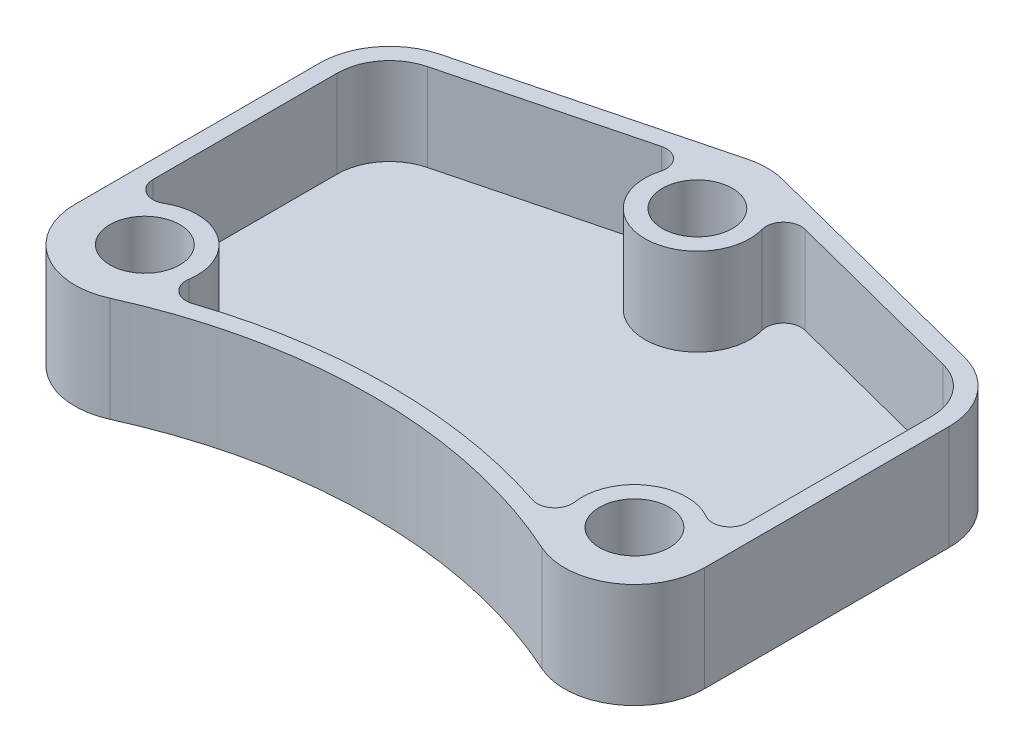
ISO-10303-21;
HEADER;
FILE_DESCRIPTION(('STEP AP214'),'2;1');
FILE_NAME('part.step','',(''),(''),'','','');
FILE_SCHEMA(('AUTOMOTIVE_DESIGN { 1 0 10303 214 1 1 1 1 }'));
ENDSEC;
DATA;
#1=APPLICATION_CONTEXT('core data for automotive mechanical design processes');
#2=APPLICATION_PROTOCOL_DEFINITION('international standard','automotive_design',2000,#1);
#3=PRODUCT_CONTEXT('',#1,'mechanical');
#4=PRODUCT('Part','Part','',(#3));
#5=PRODUCT_RELATED_PRODUCT_CATEGORY('part','',(#4));
#6=PRODUCT_DEFINITION_FORMATION('','',#4);
#7=PRODUCT_DEFINITION_CONTEXT('part definition',#1,'design');
#8=PRODUCT_DEFINITION('design','',#6,#7);
#9=PRODUCT_DEFINITION_SHAPE('','',#8);
#10=(LENGTH_UNIT() NAMED_UNIT(*) SI_UNIT(.MILLI.,.METRE.));
#11=(NAMED_UNIT(*) PLANE_ANGLE_UNIT() SI_UNIT($,.RADIAN.));
#12=(NAMED_UNIT(*) SI_UNIT($,.STERADIAN.) SOLID_ANGLE_UNIT());
#13=UNCERTAINTY_MEASURE_WITH_UNIT(LENGTH_MEASURE(1.E-05),#10,'distance_accuracy_value','');
#14=(GEOMETRIC_REPRESENTATION_CONTEXT(3) GLOBAL_UNCERTAINTY_ASSIGNED_CONTEXT((#13)) GLOBAL_UNIT_ASSIGNED_CONTEXT((#10,
#11,#12)) REPRESENTATION_CONTEXT('',''));
#15=CARTESIAN_POINT('',(0.,0.,0.));
#16=DIRECTION('',(0.,0.,1.));
#17=DIRECTION('',(1.,0.,0.));
#18=AXIS2_PLACEMENT_3D('',#15,#16,#17);
#19=CARTESIAN_POINT('',(-70.,30.,18.));
#20=DIRECTION('',(0.,1.,0.));
#21=DIRECTION('',(0.,0.,1.));
#22=AXIS2_PLACEMENT_3D('',#19,#20,#21);
#23=PLANE('',#22);
#24=CARTESIAN_POINT('',(70.,30.,88.));
#25=DIRECTION('',(0.,1.,0.));
#26=DIRECTION('',(0.,0.,1.));
#27=AXIS2_PLACEMENT_3D('',#24,#25,#26);
#28=CIRCLE('',#27,9.99999999999999);
#29=CARTESIAN_POINT('',(70.,30.,98.));
#30=VERTEX_POINT('',#29);
#31=EDGE_CURVE('E240',#30,#30,#28,.T.);
#32=ORIENTED_EDGE('',*,*,#31,.F.);
#33=EDGE_LOOP('',(#32));
#34=FACE_BOUND('',#33,.T.);
#35=CARTESIAN_POINT('',(0.,30.,0.));
#36=DIRECTION('',(0.,1.,0.));
#37=DIRECTION('',(0.,0.,1.));
#38=AXIS2_PLACEMENT_3D('',#35,#36,#37);
#39=CIRCLE('',#38,10.);
#40=CARTESIAN_POINT('',(0.,30.,10.));
#41=VERTEX_POINT('',#40);
#42=EDGE_CURVE('E163',#41,#41,#39,.T.);
#43=ORIENTED_EDGE('',*,*,#42,.F.);
#44=EDGE_LOOP('',(#43));
#45=FACE_BOUND('',#44,.T.);
#46=CARTESIAN_POINT('',(-70.,30.,18.));
#47=DIRECTION('',(0.,1.,0.));
#48=DIRECTION('',(0.,0.,1.));
#49=AXIS2_PLACEMENT_3D('',#46,#47,#48);
#50=CIRCLE('',#49,20.);
#51=CARTESIAN_POINT('',(-74.9808207962124,30.,-1.36985865193699));
#52=VERTEX_POINT('',#51);
#53=CARTESIAN_POINT('',(-90.,30.,18.));
#54=VERTEX_POINT('',#53);
#55=EDGE_CURVE('E179',#52,#54,#50,.T.);
#56=ORIENTED_EDGE('',*,*,#55,.T.);
#57=DIRECTION('',(0.,0.,1.));
#58=VECTOR('',#57,1.);
#59=CARTESIAN_POINT('',(-90.,30.,18.));
#60=LINE('',#59,#58);
#61=CARTESIAN_POINT('',(-90.,30.,88.));
#62=VERTEX_POINT('',#61);
#63=EDGE_CURVE('E109',#54,#62,#60,.T.);
#64=ORIENTED_EDGE('',*,*,#63,.T.);
#65=CARTESIAN_POINT('',(-70.,30.,88.));
#66=DIRECTION('',(0.,1.,0.));
#67=DIRECTION('',(0.,0.,1.));
#68=AXIS2_PLACEMENT_3D('',#65,#66,#67);
#69=CIRCLE('',#68,20.);
#70=CARTESIAN_POINT('',(-61.7647058823529,30.,106.225803982153));
#71=VERTEX_POINT('',#70);
#72=EDGE_CURVE('E203',#62,#71,#69,.T.);
#73=ORIENTED_EDGE('',*,*,#72,.T.);
#74=CARTESIAN_POINT('',(0.,30.,242.919333848297));
#75=DIRECTION('',(0.,-1.,0.));
#76=DIRECTION('',(0.,0.,-1.));
#77=AXIS2_PLACEMENT_3D('',#74,#75,#76);
#78=CIRCLE('',#77,150.);
#79=CARTESIAN_POINT('',(61.7647058823529,30.,106.225803982153));
#80=VERTEX_POINT('',#79);
#81=EDGE_CURVE('E219',#71,#80,#78,.T.);
#82=ORIENTED_EDGE('',*,*,#81,.T.);
#83=CARTESIAN_POINT('',(70.,30.,88.));
#84=DIRECTION('',(0.,1.,0.));
#85=DIRECTION('',(0.,0.,1.));
#86=AXIS2_PLACEMENT_3D('',#83,#84,#85);
#87=CIRCLE('',#86,20.);
#88=CARTESIAN_POINT('',(90.,30.,88.));
#89=VERTEX_POINT('',#88);
#90=EDGE_CURVE('E220',#80,#89,#87,.T.);
#91=ORIENTED_EDGE('',*,*,#90,.T.);
#92=DIRECTION('',(0.,0.,-1.));
#93=VECTOR('',#92,1.);
#94=CARTESIAN_POINT('',(90.,30.,18.));
#95=LINE('',#94,#93);
#96=CARTESIAN_POINT('',(90.,30.,18.));
#97=VERTEX_POINT('',#96);
#98=EDGE_CURVE('E218',#89,#97,#95,.T.);
#99=ORIENTED_EDGE('',*,*,#98,.T.);
#100=CARTESIAN_POINT('',(70.,30.,18.));
#101=DIRECTION('',(0.,1.,0.));
#102=DIRECTION('',(0.,0.,-1.));
#103=AXIS2_PLACEMENT_3D('',#100,#101,#102);
#104=CIRCLE('',#103,20.);
#105=CARTESIAN_POINT('',(74.9808207962124,30.,-1.36985865193699));
#106=VERTEX_POINT('',#105);
#107=EDGE_CURVE('E137',#97,#106,#104,.T.);
#108=ORIENTED_EDGE('',*,*,#107,.T.);
#109=DIRECTION('',(-0.96849293259685,0.,-0.249041039810618));
#110=VECTOR('',#109,1.);
#111=CARTESIAN_POINT('',(74.9808207962124,30.,-1.36985865193699));
#112=LINE('',#111,#110);
#113=CARTESIAN_POINT('',(4.98082079621237,30.,-19.369858651937));
#114=VERTEX_POINT('',#113);
#115=EDGE_CURVE('E135',#106,#114,#112,.T.);
#116=ORIENTED_EDGE('',*,*,#115,.T.);
#117=CARTESIAN_POINT('',(0.,30.,0.));
#118=DIRECTION('',(0.,1.,0.));
#119=DIRECTION('',(0.,0.,1.));
#120=AXIS2_PLACEMENT_3D('',#117,#118,#119);
#121=CIRCLE('',#120,20.);
#122=CARTESIAN_POINT('',(-4.98082079621237,30.,-19.369858651937));
#123=VERTEX_POINT('',#122);
#124=EDGE_CURVE('E138',#114,#123,#121,.T.);
#125=ORIENTED_EDGE('',*,*,#124,.T.);
#126=DIRECTION('',(-0.96849293259685,0.,0.249041039810618));
#127=VECTOR('',#126,1.);
#128=CARTESIAN_POINT('',(-74.9808207962124,30.,-1.36985865193699));
#129=LINE('',#128,#127);
#130=EDGE_CURVE('E64',#123,#52,#129,.T.);
#131=ORIENTED_EDGE('',*,*,#130,.T.);
#132=EDGE_LOOP('',(#56,#64,#73,#82,#91,#99,#108,#116,#125,#131));
#133=FACE_BOUND('',#132,.T.);
#134=CARTESIAN_POINT('',(-70.,30.,88.));
#135=DIRECTION('',(0.,1.,0.));
#136=DIRECTION('',(0.,0.,1.));
#137=AXIS2_PLACEMENT_3D('',#134,#135,#136);
#138=CIRCLE('',#137,9.99999999999999);
#139=CARTESIAN_POINT('',(-70.,30.,98.));
#140=VERTEX_POINT('',#139);
#141=EDGE_CURVE('E233',#140,#140,#138,.T.);
#142=ORIENTED_EDGE('',*,*,#141,.F.);
#143=EDGE_LOOP('',(#142));
#144=FACE_BOUND('',#143,.T.);
#145=CARTESIAN_POINT('',(19.2652000583974,30.,-5.37141198475075));
#146=DIRECTION('',(0.,1.,0.));
#147=DIRECTION('',(0.,0.,1.));
#148=AXIS2_PLACEMENT_3D('',#145,#146,#147);
#149=CIRCLE('',#148,5.);
#150=CARTESIAN_POINT('',(20.5104052574505,30.,-10.213876647735));
#151=VERTEX_POINT('',#150);
#152=CARTESIAN_POINT('',(14.4489000437981,30.,-4.02855898856307));
#153=VERTEX_POINT('',#152);
#154=EDGE_CURVE('E53',#151,#153,#149,.T.);
#155=ORIENTED_EDGE('',*,*,#154,.F.);
#156=DIRECTION('',(-0.96849293259685,0.,-0.249041039810618));
#157=VECTOR('',#156,1.);
#158=CARTESIAN_POINT('',(73.7356155971593,30.,3.47260601104726));
#159=LINE('',#158,#157);
#160=CARTESIAN_POINT('',(73.7356155971593,30.,3.47260601104726));
#161=VERTEX_POINT('',#160);
#162=EDGE_CURVE('E295',#161,#151,#159,.T.);
#163=ORIENTED_EDGE('',*,*,#162,.F.);
#164=CARTESIAN_POINT('',(70.,30.,18.));
#165=DIRECTION('',(0.,1.,0.));
#166=DIRECTION('',(0.,0.,1.));
#167=AXIS2_PLACEMENT_3D('',#164,#165,#166);
#168=CIRCLE('',#167,15.);
#169=CARTESIAN_POINT('',(85.,30.,18.));
#170=VERTEX_POINT('',#169);
#171=EDGE_CURVE('E297',#170,#161,#168,.T.);
#172=ORIENTED_EDGE('',*,*,#171,.F.);
#173=DIRECTION('',(0.,0.,-1.));
#174=VECTOR('',#173,1.);
#175=CARTESIAN_POINT('',(85.,30.,70.6794919243112));
#176=LINE('',#175,#174);
#177=CARTESIAN_POINT('',(85.,30.,70.6794919243112));
#178=VERTEX_POINT('',#177);
#179=EDGE_CURVE('E296',#178,#170,#176,.T.);
#180=ORIENTED_EDGE('',*,*,#179,.F.);
#181=CARTESIAN_POINT('',(80.,30.,70.6794919243112));
#182=DIRECTION('',(0.,1.,0.));
#183=DIRECTION('',(0.,0.,1.));
#184=AXIS2_PLACEMENT_3D('',#181,#182,#183);
#185=CIRCLE('',#184,5.00000000000001);
#186=CARTESIAN_POINT('',(77.5,30.,75.0096189432334));
#187=VERTEX_POINT('',#186);
#188=EDGE_CURVE('E305',#187,#178,#185,.T.);
#189=ORIENTED_EDGE('',*,*,#188,.F.);
#190=CARTESIAN_POINT('',(70.,30.,88.));
#191=DIRECTION('',(0.,-1.,0.));
#192=DIRECTION('',(0.,0.,1.));
#193=AXIS2_PLACEMENT_3D('',#190,#191,#192);
#194=CIRCLE('',#193,15.);
#195=CARTESIAN_POINT('',(55.1705641207694,30.,90.255622198815));
#196=VERTEX_POINT('',#195);
#197=EDGE_CURVE('E304',#196,#187,#194,.T.);
#198=ORIENTED_EDGE('',*,*,#197,.F.);
#199=CARTESIAN_POINT('',(50.2274188276925,30.,91.0074962650867));
#200=DIRECTION('',(0.,1.,0.));
#201=DIRECTION('',(0.,0.,1.));
#202=AXIS2_PLACEMENT_3D('',#199,#200,#201);
#203=CIRCLE('',#202,5.);
#204=CARTESIAN_POINT('',(48.6578119893271,30.,95.754741189562));
#205=VERTEX_POINT('',#204);
#206=EDGE_CURVE('E306',#205,#196,#203,.T.);
#207=ORIENTED_EDGE('',*,*,#206,.F.);
#208=CARTESIAN_POINT('',(0.,30.,242.919333848297));
#209=DIRECTION('',(0.,-1.,0.));
#210=DIRECTION('',(0.,0.,1.));
#211=AXIS2_PLACEMENT_3D('',#208,#209,#210);
#212=CIRCLE('',#211,155.);
#213=CARTESIAN_POINT('',(-48.657811989327,30.,95.754741189562));
#214=VERTEX_POINT('',#213);
#215=EDGE_CURVE('E313',#214,#205,#212,.T.);
#216=ORIENTED_EDGE('',*,*,#215,.F.);
#217=CARTESIAN_POINT('',(-50.2274188276925,30.,91.0074962650867));
#218=DIRECTION('',(0.,1.,0.));
#219=DIRECTION('',(0.,0.,1.));
#220=AXIS2_PLACEMENT_3D('',#217,#218,#219);
#221=CIRCLE('',#220,5.);
#222=CARTESIAN_POINT('',(-55.1705641207694,30.,90.255622198815));
#223=VERTEX_POINT('',#222);
#224=EDGE_CURVE('E314',#223,#214,#221,.T.);
#225=ORIENTED_EDGE('',*,*,#224,.F.);
#226=CARTESIAN_POINT('',(-70.,30.,88.));
#227=DIRECTION('',(0.,-1.,0.));
#228=DIRECTION('',(0.,0.,1.));
#229=AXIS2_PLACEMENT_3D('',#226,#227,#228);
#230=CIRCLE('',#229,15.);
#231=CARTESIAN_POINT('',(-77.5,30.,75.0096189432334));
#232=VERTEX_POINT('',#231);
#233=EDGE_CURVE('E320',#232,#223,#230,.T.);
#234=ORIENTED_EDGE('',*,*,#233,.F.);
#235=CARTESIAN_POINT('',(-80.,30.,70.6794919243112));
#236=DIRECTION('',(0.,1.,0.));
#237=DIRECTION('',(0.,0.,1.));
#238=AXIS2_PLACEMENT_3D('',#235,#236,#237);
#239=CIRCLE('',#238,5.);
#240=CARTESIAN_POINT('',(-85.,30.,70.6794919243112));
#241=VERTEX_POINT('',#240);
#242=EDGE_CURVE('E319',#241,#232,#239,.T.);
#243=ORIENTED_EDGE('',*,*,#242,.F.);
#244=DIRECTION('',(0.,0.,1.));
#245=VECTOR('',#244,1.);
#246=CARTESIAN_POINT('',(-85.,30.,18.));
#247=LINE('',#246,#245);
#248=CARTESIAN_POINT('',(-85.,30.,18.));
#249=VERTEX_POINT('',#248);
#250=EDGE_CURVE('E323',#249,#241,#247,.T.);
#251=ORIENTED_EDGE('',*,*,#250,.F.);
#252=CARTESIAN_POINT('',(-70.,30.,18.));
#253=DIRECTION('',(0.,1.,0.));
#254=DIRECTION('',(0.,0.,1.));
#255=AXIS2_PLACEMENT_3D('',#252,#253,#254);
#256=CIRCLE('',#255,15.);
#257=CARTESIAN_POINT('',(-73.7356155971593,30.,3.47260601104725));
#258=VERTEX_POINT('',#257);
#259=EDGE_CURVE('E326',#258,#249,#256,.T.);
#260=ORIENTED_EDGE('',*,*,#259,.F.);
#261=DIRECTION('',(-0.96849293259685,0.,0.249041039810618));
#262=VECTOR('',#261,1.);
#263=CARTESIAN_POINT('',(-20.5104052574505,30.,-10.213876647735));
#264=LINE('',#263,#262);
#265=CARTESIAN_POINT('',(-20.5104052574505,30.,-10.213876647735));
#266=VERTEX_POINT('',#265);
#267=EDGE_CURVE('E328',#266,#258,#264,.T.);
#268=ORIENTED_EDGE('',*,*,#267,.F.);
#269=CARTESIAN_POINT('',(-19.2652000583974,30.,-5.37141198475075));
#270=DIRECTION('',(0.,1.,0.));
#271=DIRECTION('',(0.,0.,1.));
#272=AXIS2_PLACEMENT_3D('',#269,#270,#271);
#273=CIRCLE('',#272,5.);
#274=CARTESIAN_POINT('',(-14.4489000437981,30.,-4.02855898856306));
#275=VERTEX_POINT('',#274);
#276=EDGE_CURVE('E335',#275,#266,#273,.T.);
#277=ORIENTED_EDGE('',*,*,#276,.F.);
#278=CARTESIAN_POINT('',(0.,30.,0.));
#279=DIRECTION('',(0.,-1.,0.));
#280=DIRECTION('',(0.,0.,1.));
#281=AXIS2_PLACEMENT_3D('',#278,#279,#280);
#282=CIRCLE('',#281,15.);
#283=EDGE_CURVE('E333',#153,#275,#282,.T.);
#284=ORIENTED_EDGE('',*,*,#283,.F.);
#285=EDGE_LOOP('',(#155,#163,#172,#180,#189,#198,#207,#216,#225,#234,#243,#251,#260,#268,#277,#284));
#286=FACE_BOUND('',#285,.T.);
#287=ADVANCED_FACE('F39',(#34,#45,#133,#144,#286),#23,.T.);
#288=CARTESIAN_POINT('',(-70.,0.,18.));
#289=DIRECTION('',(0.,1.,0.));
#290=DIRECTION('',(0.,0.,1.));
#291=AXIS2_PLACEMENT_3D('',#288,#289,#290);
#292=PLANE('',#291);
#293=CARTESIAN_POINT('',(-70.,0.,18.));
#294=DIRECTION('',(0.,1.,0.));
#295=DIRECTION('',(0.,0.,1.));
#296=AXIS2_PLACEMENT_3D('',#293,#294,#295);
#297=CIRCLE('',#296,20.);
#298=CARTESIAN_POINT('',(-74.9808207962124,0.,-1.36985865193699));
#299=VERTEX_POINT('',#298);
#300=CARTESIAN_POINT('',(-90.,0.,18.));
#301=VERTEX_POINT('',#300);
#302=EDGE_CURVE('E159',#299,#301,#297,.T.);
#303=ORIENTED_EDGE('',*,*,#302,.F.);
#304=DIRECTION('',(-0.96849293259685,0.,0.249041039810618));
#305=VECTOR('',#304,1.);
#306=CARTESIAN_POINT('',(-74.9808207962124,0.,-1.36985865193699));
#307=LINE('',#306,#305);
#308=CARTESIAN_POINT('',(-4.98082079621237,0.,-19.369858651937));
#309=VERTEX_POINT('',#308);
#310=EDGE_CURVE('E105',#309,#299,#307,.T.);
#311=ORIENTED_EDGE('',*,*,#310,.F.);
#312=CARTESIAN_POINT('',(0.,0.,0.));
#313=DIRECTION('',(0.,1.,0.));
#314=DIRECTION('',(0.,0.,1.));
#315=AXIS2_PLACEMENT_3D('',#312,#313,#314);
#316=CIRCLE('',#315,20.);
#317=CARTESIAN_POINT('',(4.98082079621237,0.,-19.369858651937));
#318=VERTEX_POINT('',#317);
#319=EDGE_CURVE('E180',#318,#309,#316,.T.);
#320=ORIENTED_EDGE('',*,*,#319,.F.);
#321=DIRECTION('',(-0.96849293259685,0.,-0.249041039810618));
#322=VECTOR('',#321,1.);
#323=CARTESIAN_POINT('',(74.9808207962124,0.,-1.36985865193699));
#324=LINE('',#323,#322);
#325=CARTESIAN_POINT('',(74.9808207962124,0.,-1.36985865193699));
#326=VERTEX_POINT('',#325);
#327=EDGE_CURVE('E146',#326,#318,#324,.T.);
#328=ORIENTED_EDGE('',*,*,#327,.F.);
#329=CARTESIAN_POINT('',(70.,0.,18.));
#330=DIRECTION('',(0.,1.,0.));
#331=DIRECTION('',(0.,0.,-1.));
#332=AXIS2_PLACEMENT_3D('',#329,#330,#331);
#333=CIRCLE('',#332,20.);
#334=CARTESIAN_POINT('',(90.,0.,18.));
#335=VERTEX_POINT('',#334);
#336=EDGE_CURVE('E171',#335,#326,#333,.T.);
#337=ORIENTED_EDGE('',*,*,#336,.F.);
#338=DIRECTION('',(0.,0.,-1.));
#339=VECTOR('',#338,1.);
#340=CARTESIAN_POINT('',(90.,0.,18.));
#341=LINE('',#340,#339);
#342=CARTESIAN_POINT('',(90.,0.,88.));
#343=VERTEX_POINT('',#342);
#344=EDGE_CURVE('E175',#343,#335,#341,.T.);
#345=ORIENTED_EDGE('',*,*,#344,.F.);
#346=CARTESIAN_POINT('',(70.,0.,88.));
#347=DIRECTION('',(0.,1.,0.));
#348=DIRECTION('',(0.,0.,1.));
#349=AXIS2_PLACEMENT_3D('',#346,#347,#348);
#350=CIRCLE('',#349,20.);
#351=CARTESIAN_POINT('',(61.7647058823529,0.,106.225803982153));
#352=VERTEX_POINT('',#351);
#353=EDGE_CURVE('E168',#352,#343,#350,.T.);
#354=ORIENTED_EDGE('',*,*,#353,.F.);
#355=CARTESIAN_POINT('',(0.,0.,242.919333848297));
#356=DIRECTION('',(0.,-1.,0.));
#357=DIRECTION('',(0.,0.,-1.));
#358=AXIS2_PLACEMENT_3D('',#355,#356,#357);
#359=CIRCLE('',#358,150.);
#360=CARTESIAN_POINT('',(-61.7647058823529,0.,106.225803982153));
#361=VERTEX_POINT('',#360);
#362=EDGE_CURVE('E169',#361,#352,#359,.T.);
#363=ORIENTED_EDGE('',*,*,#362,.F.);
#364=CARTESIAN_POINT('',(-70.,0.,88.));
#365=DIRECTION('',(0.,1.,0.));
#366=DIRECTION('',(0.,0.,1.));
#367=AXIS2_PLACEMENT_3D('',#364,#365,#366);
#368=CIRCLE('',#367,20.);
#369=CARTESIAN_POINT('',(-90.,0.,88.));
#370=VERTEX_POINT('',#369);
#371=EDGE_CURVE('E167',#370,#361,#368,.T.);
#372=ORIENTED_EDGE('',*,*,#371,.F.);
#373=DIRECTION('',(0.,0.,1.));
#374=VECTOR('',#373,1.);
#375=CARTESIAN_POINT('',(-90.,0.,18.));
#376=LINE('',#375,#374);
#377=EDGE_CURVE('E162',#301,#370,#376,.T.);
#378=ORIENTED_EDGE('',*,*,#377,.F.);
#379=EDGE_LOOP('',(#303,#311,#320,#328,#337,#345,#354,#363,#372,#378));
#380=FACE_BOUND('',#379,.T.);
#381=CARTESIAN_POINT('',(0.,0.,0.));
#382=DIRECTION('',(0.,1.,0.));
#383=DIRECTION('',(0.,0.,1.));
#384=AXIS2_PLACEMENT_3D('',#381,#382,#383);
#385=CIRCLE('',#384,10.);
#386=CARTESIAN_POINT('',(0.,0.,10.));
#387=VERTEX_POINT('',#386);
#388=EDGE_CURVE('E229',#387,#387,#385,.T.);
#389=ORIENTED_EDGE('',*,*,#388,.T.);
#390=EDGE_LOOP('',(#389));
#391=FACE_BOUND('',#390,.T.);
#392=CARTESIAN_POINT('',(-70.,0.,88.));
#393=DIRECTION('',(0.,1.,0.));
#394=DIRECTION('',(0.,0.,1.));
#395=AXIS2_PLACEMENT_3D('',#392,#393,#394);
#396=CIRCLE('',#395,9.99999999999999);
#397=CARTESIAN_POINT('',(-70.,0.,98.));
#398=VERTEX_POINT('',#397);
#399=EDGE_CURVE('E232',#398,#398,#396,.T.);
#400=ORIENTED_EDGE('',*,*,#399,.T.);
#401=EDGE_LOOP('',(#400));
#402=FACE_BOUND('',#401,.T.);
#403=CARTESIAN_POINT('',(70.,0.,88.));
#404=DIRECTION('',(0.,1.,0.));
#405=DIRECTION('',(0.,0.,1.));
#406=AXIS2_PLACEMENT_3D('',#403,#404,#405);
#407=CIRCLE('',#406,9.99999999999999);
#408=CARTESIAN_POINT('',(70.,0.,98.));
#409=VERTEX_POINT('',#408);
#410=EDGE_CURVE('E238',#409,#409,#407,.T.);
#411=ORIENTED_EDGE('',*,*,#410,.T.);
#412=EDGE_LOOP('',(#411));
#413=FACE_BOUND('',#412,.T.);
#414=ADVANCED_FACE('F202',(#380,#391,#402,#413),#292,.F.);
#415=CARTESIAN_POINT('',(-70.,30.,18.));
#416=DIRECTION('',(0.,-1.,0.));
#417=DIRECTION('',(0.,0.,-1.));
#418=AXIS2_PLACEMENT_3D('',#415,#416,#417);
#419=CYLINDRICAL_SURFACE('',#418,20.);
#420=ORIENTED_EDGE('',*,*,#302,.T.);
#421=DIRECTION('',(0.,-1.,0.));
#422=VECTOR('',#421,1.);
#423=CARTESIAN_POINT('',(-90.,30.,18.));
#424=LINE('',#423,#422);
#425=EDGE_CURVE('E11',#54,#301,#424,.T.);
#426=ORIENTED_EDGE('',*,*,#425,.F.);
#427=ORIENTED_EDGE('',*,*,#55,.F.);
#428=DIRECTION('',(0.,-1.,0.));
#429=VECTOR('',#428,1.);
#430=CARTESIAN_POINT('',(-74.9808207962124,30.,-1.36985865193699));
#431=LINE('',#430,#429);
#432=EDGE_CURVE('E156',#52,#299,#431,.T.);
#433=ORIENTED_EDGE('',*,*,#432,.T.);
#434=EDGE_LOOP('',(#420,#426,#427,#433));
#435=FACE_BOUND('',#434,.T.);
#436=ADVANCED_FACE('F41',(#435),#419,.T.);
#437=CARTESIAN_POINT('',(-90.,30.,18.));
#438=DIRECTION('',(1.,0.,0.));
#439=DIRECTION('',(0.,0.,-1.));
#440=AXIS2_PLACEMENT_3D('',#437,#438,#439);
#441=PLANE('',#440);
#442=ORIENTED_EDGE('',*,*,#377,.T.);
#443=DIRECTION('',(0.,-1.,0.));
#444=VECTOR('',#443,1.);
#445=CARTESIAN_POINT('',(-90.,30.,88.));
#446=LINE('',#445,#444);
#447=EDGE_CURVE('E50',#62,#370,#446,.T.);
#448=ORIENTED_EDGE('',*,*,#447,.F.);
#449=ORIENTED_EDGE('',*,*,#63,.F.);
#450=ORIENTED_EDGE('',*,*,#425,.T.);
#451=EDGE_LOOP('',(#442,#448,#449,#450));
#452=FACE_BOUND('',#451,.T.);
#453=ADVANCED_FACE('F564',(#452),#441,.F.);
#454=CARTESIAN_POINT('',(-70.,30.,88.));
#455=DIRECTION('',(0.,-1.,0.));
#456=DIRECTION('',(0.,0.,-1.));
#457=AXIS2_PLACEMENT_3D('',#454,#455,#456);
#458=CYLINDRICAL_SURFACE('',#457,20.);
#459=ORIENTED_EDGE('',*,*,#371,.T.);
#460=DIRECTION('',(0.,-1.,0.));
#461=VECTOR('',#460,1.);
#462=CARTESIAN_POINT('',(-61.7647058823529,30.,106.225803982153));
#463=LINE('',#462,#461);
#464=EDGE_CURVE('E191',#71,#361,#463,.T.);
#465=ORIENTED_EDGE('',*,*,#464,.F.);
#466=ORIENTED_EDGE('',*,*,#72,.F.);
#467=ORIENTED_EDGE('',*,*,#447,.T.);
#468=EDGE_LOOP('',(#459,#465,#466,#467));
#469=FACE_BOUND('',#468,.T.);
#470=ADVANCED_FACE('F200',(#469),#458,.T.);
#471=CARTESIAN_POINT('',(0.,30.,242.919333848297));
#472=DIRECTION('',(0.,-1.,0.));
#473=DIRECTION('',(0.,0.,-1.));
#474=AXIS2_PLACEMENT_3D('',#471,#472,#473);
#475=CYLINDRICAL_SURFACE('',#474,150.);
#476=ORIENTED_EDGE('',*,*,#362,.T.);
#477=DIRECTION('',(0.,-1.,0.));
#478=VECTOR('',#477,1.);
#479=CARTESIAN_POINT('',(61.7647058823529,30.,106.225803982153));
#480=LINE('',#479,#478);
#481=EDGE_CURVE('E188',#80,#352,#480,.T.);
#482=ORIENTED_EDGE('',*,*,#481,.F.);
#483=ORIENTED_EDGE('',*,*,#81,.F.);
#484=ORIENTED_EDGE('',*,*,#464,.T.);
#485=EDGE_LOOP('',(#476,#482,#483,#484));
#486=FACE_BOUND('',#485,.T.);
#487=ADVANCED_FACE('F211',(#486),#475,.F.);
#488=CARTESIAN_POINT('',(70.,30.,88.));
#489=DIRECTION('',(0.,-1.,0.));
#490=DIRECTION('',(0.,0.,-1.));
#491=AXIS2_PLACEMENT_3D('',#488,#489,#490);
#492=CYLINDRICAL_SURFACE('',#491,20.);
#493=ORIENTED_EDGE('',*,*,#353,.T.);
#494=DIRECTION('',(0.,-1.,0.));
#495=VECTOR('',#494,1.);
#496=CARTESIAN_POINT('',(90.,30.,88.));
#497=LINE('',#496,#495);
#498=EDGE_CURVE('E190',#89,#343,#497,.T.);
#499=ORIENTED_EDGE('',*,*,#498,.F.);
#500=ORIENTED_EDGE('',*,*,#90,.F.);
#501=ORIENTED_EDGE('',*,*,#481,.T.);
#502=EDGE_LOOP('',(#493,#499,#500,#501));
#503=FACE_BOUND('',#502,.T.);
#504=ADVANCED_FACE('F214',(#503),#492,.T.);
#505=CARTESIAN_POINT('',(90.,30.,18.));
#506=DIRECTION('',(-1.,0.,0.));
#507=DIRECTION('',(0.,0.,1.));
#508=AXIS2_PLACEMENT_3D('',#505,#506,#507);
#509=PLANE('',#508);
#510=ORIENTED_EDGE('',*,*,#344,.T.);
#511=DIRECTION('',(0.,-1.,0.));
#512=VECTOR('',#511,1.);
#513=CARTESIAN_POINT('',(90.,30.,18.));
#514=LINE('',#513,#512);
#515=EDGE_CURVE('E184',#97,#335,#514,.T.);
#516=ORIENTED_EDGE('',*,*,#515,.F.);
#517=ORIENTED_EDGE('',*,*,#98,.F.);
#518=ORIENTED_EDGE('',*,*,#498,.T.);
#519=EDGE_LOOP('',(#510,#516,#517,#518));
#520=FACE_BOUND('',#519,.T.);
#521=ADVANCED_FACE('F553',(#520),#509,.F.);
#522=CARTESIAN_POINT('',(70.,30.,18.));
#523=DIRECTION('',(0.,-1.,0.));
#524=DIRECTION('',(0.,0.,-1.));
#525=AXIS2_PLACEMENT_3D('',#522,#523,#524);
#526=CYLINDRICAL_SURFACE('',#525,20.);
#527=ORIENTED_EDGE('',*,*,#336,.T.);
#528=DIRECTION('',(0.,-1.,0.));
#529=VECTOR('',#528,1.);
#530=CARTESIAN_POINT('',(74.9808207962124,30.,-1.36985865193699));
#531=LINE('',#530,#529);
#532=EDGE_CURVE('E151',#106,#326,#531,.T.);
#533=ORIENTED_EDGE('',*,*,#532,.F.);
#534=ORIENTED_EDGE('',*,*,#107,.F.);
#535=ORIENTED_EDGE('',*,*,#515,.T.);
#536=EDGE_LOOP('',(#527,#533,#534,#535));
#537=FACE_BOUND('',#536,.T.);
#538=ADVANCED_FACE('F555',(#537),#526,.T.);
#539=CARTESIAN_POINT('',(74.9808207962124,30.,-1.36985865193699));
#540=DIRECTION('',(-0.249041039810619,0.,0.96849293259685));
#541=DIRECTION('',(0.96849293259685,0.,0.249041039810619));
#542=AXIS2_PLACEMENT_3D('',#539,#540,#541);
#543=PLANE('',#542);
#544=ORIENTED_EDGE('',*,*,#327,.T.);
#545=DIRECTION('',(0.,-1.,0.));
#546=VECTOR('',#545,1.);
#547=CARTESIAN_POINT('',(4.98082079621237,30.,-19.369858651937));
#548=LINE('',#547,#546);
#549=EDGE_CURVE('E144',#114,#318,#548,.T.);
#550=ORIENTED_EDGE('',*,*,#549,.F.);
#551=ORIENTED_EDGE('',*,*,#115,.F.);
#552=ORIENTED_EDGE('',*,*,#532,.T.);
#553=EDGE_LOOP('',(#544,#550,#551,#552));
#554=FACE_BOUND('',#553,.T.);
#555=ADVANCED_FACE('F148',(#554),#543,.F.);
#556=CARTESIAN_POINT('',(0.,30.,0.));
#557=DIRECTION('',(0.,-1.,0.));
#558=DIRECTION('',(0.,0.,-1.));
#559=AXIS2_PLACEMENT_3D('',#556,#557,#558);
#560=CYLINDRICAL_SURFACE('',#559,20.);
#561=ORIENTED_EDGE('',*,*,#319,.T.);
#562=DIRECTION('',(0.,-1.,0.));
#563=VECTOR('',#562,1.);
#564=CARTESIAN_POINT('',(-4.98082079621237,30.,-19.369858651937));
#565=LINE('',#564,#563);
#566=EDGE_CURVE('E155',#123,#309,#565,.T.);
#567=ORIENTED_EDGE('',*,*,#566,.F.);
#568=ORIENTED_EDGE('',*,*,#124,.F.);
#569=ORIENTED_EDGE('',*,*,#549,.T.);
#570=EDGE_LOOP('',(#561,#567,#568,#569));
#571=FACE_BOUND('',#570,.T.);
#572=ADVANCED_FACE('F152',(#571),#560,.T.);
#573=CARTESIAN_POINT('',(-74.9808207962124,30.,-1.36985865193699));
#574=DIRECTION('',(0.249041039810619,0.,0.96849293259685));
#575=DIRECTION('',(0.96849293259685,0.,-0.249041039810619));
#576=AXIS2_PLACEMENT_3D('',#573,#574,#575);
#577=PLANE('',#576);
#578=ORIENTED_EDGE('',*,*,#310,.T.);
#579=ORIENTED_EDGE('',*,*,#432,.F.);
#580=ORIENTED_EDGE('',*,*,#130,.F.);
#581=ORIENTED_EDGE('',*,*,#566,.T.);
#582=EDGE_LOOP('',(#578,#579,#580,#581));
#583=FACE_BOUND('',#582,.T.);
#584=ADVANCED_FACE('F544',(#583),#577,.F.);
#585=CARTESIAN_POINT('',(0.,30.,0.));
#586=DIRECTION('',(0.,-1.,0.));
#587=DIRECTION('',(0.,0.,-1.));
#588=AXIS2_PLACEMENT_3D('',#585,#586,#587);
#589=CYLINDRICAL_SURFACE('',#588,10.);
#590=ORIENTED_EDGE('',*,*,#42,.T.);
#591=EDGE_LOOP('',(#590));
#592=FACE_BOUND('',#591,.T.);
#593=ORIENTED_EDGE('',*,*,#388,.F.);
#594=EDGE_LOOP('',(#593));
#595=FACE_BOUND('',#594,.T.);
#596=ADVANCED_FACE('F545',(#592,#595),#589,.F.);
#597=CARTESIAN_POINT('',(-70.,30.,88.));
#598=DIRECTION('',(0.,-1.,0.));
#599=DIRECTION('',(0.,0.,-1.));
#600=AXIS2_PLACEMENT_3D('',#597,#598,#599);
#601=CYLINDRICAL_SURFACE('',#600,9.99999999999999);
#602=ORIENTED_EDGE('',*,*,#141,.T.);
#603=EDGE_LOOP('',(#602));
#604=FACE_BOUND('',#603,.T.);
#605=ORIENTED_EDGE('',*,*,#399,.F.);
#606=EDGE_LOOP('',(#605));
#607=FACE_BOUND('',#606,.T.);
#608=ADVANCED_FACE('F638',(#604,#607),#601,.F.);
#609=CARTESIAN_POINT('',(70.,30.,88.));
#610=DIRECTION('',(0.,-1.,0.));
#611=DIRECTION('',(0.,0.,-1.));
#612=AXIS2_PLACEMENT_3D('',#609,#610,#611);
#613=CYLINDRICAL_SURFACE('',#612,9.99999999999999);
#614=ORIENTED_EDGE('',*,*,#31,.T.);
#615=EDGE_LOOP('',(#614));
#616=FACE_BOUND('',#615,.T.);
#617=ORIENTED_EDGE('',*,*,#410,.F.);
#618=EDGE_LOOP('',(#617));
#619=FACE_BOUND('',#618,.T.);
#620=ADVANCED_FACE('F644',(#616,#619),#613,.F.);
#621=CARTESIAN_POINT('',(19.2652000583974,5.,-5.37141198475075));
#622=DIRECTION('',(0.,1.,0.));
#623=DIRECTION('',(0.,0.,1.));
#624=AXIS2_PLACEMENT_3D('',#621,#622,#623);
#625=CYLINDRICAL_SURFACE('',#624,5.);
#626=ORIENTED_EDGE('',*,*,#154,.T.);
#627=DIRECTION('',(0.,1.,0.));
#628=VECTOR('',#627,1.);
#629=CARTESIAN_POINT('',(14.4489000437981,5.,-4.02855898856307));
#630=LINE('',#629,#628);
#631=CARTESIAN_POINT('',(14.4489000437981,5.,-4.02855898856307));
#632=VERTEX_POINT('',#631);
#633=EDGE_CURVE('E248',#632,#153,#630,.T.);
#634=ORIENTED_EDGE('',*,*,#633,.F.);
#635=CARTESIAN_POINT('',(19.2652000583974,5.,-5.37141198475075));
#636=DIRECTION('',(0.,1.,0.));
#637=DIRECTION('',(0.,0.,1.));
#638=AXIS2_PLACEMENT_3D('',#635,#636,#637);
#639=CIRCLE('',#638,5.);
#640=CARTESIAN_POINT('',(20.5104052574505,5.,-10.213876647735));
#641=VERTEX_POINT('',#640);
#642=EDGE_CURVE('E293',#641,#632,#639,.T.);
#643=ORIENTED_EDGE('',*,*,#642,.F.);
#644=DIRECTION('',(0.,1.,0.));
#645=VECTOR('',#644,1.);
#646=CARTESIAN_POINT('',(20.5104052574505,5.,-10.213876647735));
#647=LINE('',#646,#645);
#648=EDGE_CURVE('E244',#641,#151,#647,.T.);
#649=ORIENTED_EDGE('',*,*,#648,.T.);
#650=EDGE_LOOP('',(#626,#634,#643,#649));
#651=FACE_BOUND('',#650,.T.);
#652=ADVANCED_FACE('F395',(#651),#625,.F.);
#653=CARTESIAN_POINT('',(73.7356155971593,5.,3.47260601104726));
#654=DIRECTION('',(0.249041039810618,0.,-0.96849293259685));
#655=DIRECTION('',(-0.96849293259685,0.,-0.249041039810618));
#656=AXIS2_PLACEMENT_3D('',#653,#654,#655);
#657=PLANE('',#656);
#658=ORIENTED_EDGE('',*,*,#162,.T.);
#659=ORIENTED_EDGE('',*,*,#648,.F.);
#660=DIRECTION('',(-0.96849293259685,0.,-0.249041039810618));
#661=VECTOR('',#660,1.);
#662=CARTESIAN_POINT('',(73.7356155971593,5.,3.47260601104726));
#663=LINE('',#662,#661);
#664=CARTESIAN_POINT('',(73.7356155971593,5.,3.47260601104726));
#665=VERTEX_POINT('',#664);
#666=EDGE_CURVE('E247',#665,#641,#663,.T.);
#667=ORIENTED_EDGE('',*,*,#666,.F.);
#668=DIRECTION('',(0.,1.,0.));
#669=VECTOR('',#668,1.);
#670=CARTESIAN_POINT('',(73.7356155971593,5.,3.47260601104726));
#671=LINE('',#670,#669);
#672=EDGE_CURVE('E286',#665,#161,#671,.T.);
#673=ORIENTED_EDGE('',*,*,#672,.T.);
#674=EDGE_LOOP('',(#658,#659,#667,#673));
#675=FACE_BOUND('',#674,.T.);
#676=ADVANCED_FACE('F428',(#675),#657,.F.);
#677=CARTESIAN_POINT('',(70.,5.,18.));
#678=DIRECTION('',(0.,1.,0.));
#679=DIRECTION('',(0.,0.,1.));
#680=AXIS2_PLACEMENT_3D('',#677,#678,#679);
#681=CYLINDRICAL_SURFACE('',#680,15.);
#682=ORIENTED_EDGE('',*,*,#171,.T.);
#683=ORIENTED_EDGE('',*,*,#672,.F.);
#684=CARTESIAN_POINT('',(70.,5.,18.));
#685=DIRECTION('',(0.,1.,0.));
#686=DIRECTION('',(0.,0.,1.));
#687=AXIS2_PLACEMENT_3D('',#684,#685,#686);
#688=CIRCLE('',#687,15.);
#689=CARTESIAN_POINT('',(85.,5.,18.));
#690=VERTEX_POINT('',#689);
#691=EDGE_CURVE('E343',#690,#665,#688,.T.);
#692=ORIENTED_EDGE('',*,*,#691,.F.);
#693=DIRECTION('',(0.,1.,0.));
#694=VECTOR('',#693,1.);
#695=CARTESIAN_POINT('',(85.,5.,18.));
#696=LINE('',#695,#694);
#697=EDGE_CURVE('E283',#690,#170,#696,.T.);
#698=ORIENTED_EDGE('',*,*,#697,.T.);
#699=EDGE_LOOP('',(#682,#683,#692,#698));
#700=FACE_BOUND('',#699,.T.);
#701=ADVANCED_FACE('F433',(#700),#681,.F.);
#702=CARTESIAN_POINT('',(85.,5.,70.6794919243112));
#703=DIRECTION('',(1.,0.,0.));
#704=DIRECTION('',(0.,0.,-1.));
#705=AXIS2_PLACEMENT_3D('',#702,#703,#704);
#706=PLANE('',#705);
#707=ORIENTED_EDGE('',*,*,#179,.T.);
#708=ORIENTED_EDGE('',*,*,#697,.F.);
#709=DIRECTION('',(0.,0.,-1.));
#710=VECTOR('',#709,1.);
#711=CARTESIAN_POINT('',(85.,5.,70.6794919243112));
#712=LINE('',#711,#710);
#713=CARTESIAN_POINT('',(85.,5.,70.6794919243112));
#714=VERTEX_POINT('',#713);
#715=EDGE_CURVE('E342',#714,#690,#712,.T.);
#716=ORIENTED_EDGE('',*,*,#715,.F.);
#717=DIRECTION('',(0.,1.,0.));
#718=VECTOR('',#717,1.);
#719=CARTESIAN_POINT('',(85.,5.,70.6794919243112));
#720=LINE('',#719,#718);
#721=EDGE_CURVE('E285',#714,#178,#720,.T.);
#722=ORIENTED_EDGE('',*,*,#721,.T.);
#723=EDGE_LOOP('',(#707,#708,#716,#722));
#724=FACE_BOUND('',#723,.T.);
#725=ADVANCED_FACE('F483',(#724),#706,.F.);
#726=CARTESIAN_POINT('',(80.,5.,70.6794919243112));
#727=DIRECTION('',(0.,1.,0.));
#728=DIRECTION('',(0.,0.,1.));
#729=AXIS2_PLACEMENT_3D('',#726,#727,#728);
#730=CYLINDRICAL_SURFACE('',#729,5.00000000000001);
#731=ORIENTED_EDGE('',*,*,#188,.T.);
#732=ORIENTED_EDGE('',*,*,#721,.F.);
#733=CARTESIAN_POINT('',(80.,5.,70.6794919243112));
#734=DIRECTION('',(0.,1.,0.));
#735=DIRECTION('',(0.,0.,1.));
#736=AXIS2_PLACEMENT_3D('',#733,#734,#735);
#737=CIRCLE('',#736,5.00000000000001);
#738=CARTESIAN_POINT('',(77.5,5.,75.0096189432334));
#739=VERTEX_POINT('',#738);
#740=EDGE_CURVE('E350',#739,#714,#737,.T.);
#741=ORIENTED_EDGE('',*,*,#740,.F.);
#742=DIRECTION('',(0.,1.,0.));
#743=VECTOR('',#742,1.);
#744=CARTESIAN_POINT('',(77.5,5.,75.0096189432334));
#745=LINE('',#744,#743);
#746=EDGE_CURVE('E276',#739,#187,#745,.T.);
#747=ORIENTED_EDGE('',*,*,#746,.T.);
#748=EDGE_LOOP('',(#731,#732,#741,#747));
#749=FACE_BOUND('',#748,.T.);
#750=ADVANCED_FACE('F490',(#749),#730,.F.);
#751=CARTESIAN_POINT('',(70.,5.,88.));
#752=DIRECTION('',(0.,1.,0.));
#753=DIRECTION('',(0.,0.,1.));
#754=AXIS2_PLACEMENT_3D('',#751,#752,#753);
#755=CYLINDRICAL_SURFACE('',#754,15.);
#756=ORIENTED_EDGE('',*,*,#197,.T.);
#757=ORIENTED_EDGE('',*,*,#746,.F.);
#758=CARTESIAN_POINT('',(70.,5.,88.));
#759=DIRECTION('',(0.,-1.,0.));
#760=DIRECTION('',(0.,0.,1.));
#761=AXIS2_PLACEMENT_3D('',#758,#759,#760);
#762=CIRCLE('',#761,15.);
#763=CARTESIAN_POINT('',(55.1705641207694,5.,90.255622198815));
#764=VERTEX_POINT('',#763);
#765=EDGE_CURVE('E348',#764,#739,#762,.T.);
#766=ORIENTED_EDGE('',*,*,#765,.F.);
#767=DIRECTION('',(0.,1.,0.));
#768=VECTOR('',#767,1.);
#769=CARTESIAN_POINT('',(55.1705641207694,5.,90.255622198815));
#770=LINE('',#769,#768);
#771=EDGE_CURVE('E277',#764,#196,#770,.T.);
#772=ORIENTED_EDGE('',*,*,#771,.T.);
#773=EDGE_LOOP('',(#756,#757,#766,#772));
#774=FACE_BOUND('',#773,.T.);
#775=ADVANCED_FACE('F492',(#774),#755,.T.);
#776=CARTESIAN_POINT('',(50.2274188276925,5.,91.0074962650867));
#777=DIRECTION('',(0.,1.,0.));
#778=DIRECTION('',(0.,0.,1.));
#779=AXIS2_PLACEMENT_3D('',#776,#777,#778);
#780=CYLINDRICAL_SURFACE('',#779,5.);
#781=ORIENTED_EDGE('',*,*,#206,.T.);
#782=ORIENTED_EDGE('',*,*,#771,.F.);
#783=CARTESIAN_POINT('',(50.2274188276925,5.,91.0074962650867));
#784=DIRECTION('',(0.,1.,0.));
#785=DIRECTION('',(0.,0.,1.));
#786=AXIS2_PLACEMENT_3D('',#783,#784,#785);
#787=CIRCLE('',#786,5.);
#788=CARTESIAN_POINT('',(48.6578119893271,5.,95.754741189562));
#789=VERTEX_POINT('',#788);
#790=EDGE_CURVE('E354',#789,#764,#787,.T.);
#791=ORIENTED_EDGE('',*,*,#790,.F.);
#792=DIRECTION('',(0.,1.,0.));
#793=VECTOR('',#792,1.);
#794=CARTESIAN_POINT('',(48.6578119893271,5.,95.754741189562));
#795=LINE('',#794,#793);
#796=EDGE_CURVE('E272',#789,#205,#795,.T.);
#797=ORIENTED_EDGE('',*,*,#796,.T.);
#798=EDGE_LOOP('',(#781,#782,#791,#797));
#799=FACE_BOUND('',#798,.T.);
#800=ADVANCED_FACE('F497',(#799),#780,.F.);
#801=CARTESIAN_POINT('',(0.,5.,242.919333848297));
#802=DIRECTION('',(0.,1.,0.));
#803=DIRECTION('',(0.,0.,1.));
#804=AXIS2_PLACEMENT_3D('',#801,#802,#803);
#805=CYLINDRICAL_SURFACE('',#804,155.);
#806=ORIENTED_EDGE('',*,*,#215,.T.);
#807=ORIENTED_EDGE('',*,*,#796,.F.);
#808=CARTESIAN_POINT('',(0.,5.,242.919333848297));
#809=DIRECTION('',(0.,-1.,0.));
#810=DIRECTION('',(0.,0.,1.));
#811=AXIS2_PLACEMENT_3D('',#808,#809,#810);
#812=CIRCLE('',#811,155.);
#813=CARTESIAN_POINT('',(-48.657811989327,5.,95.754741189562));
#814=VERTEX_POINT('',#813);
#815=EDGE_CURVE('E358',#814,#789,#812,.T.);
#816=ORIENTED_EDGE('',*,*,#815,.F.);
#817=DIRECTION('',(0.,1.,0.));
#818=VECTOR('',#817,1.);
#819=CARTESIAN_POINT('',(-48.657811989327,5.,95.754741189562));
#820=LINE('',#819,#818);
#821=EDGE_CURVE('E269',#814,#214,#820,.T.);
#822=ORIENTED_EDGE('',*,*,#821,.T.);
#823=EDGE_LOOP('',(#806,#807,#816,#822));
#824=FACE_BOUND('',#823,.T.);
#825=ADVANCED_FACE('F496',(#824),#805,.T.);
#826=CARTESIAN_POINT('',(-50.2274188276925,5.,91.0074962650867));
#827=DIRECTION('',(0.,1.,0.));
#828=DIRECTION('',(0.,0.,1.));
#829=AXIS2_PLACEMENT_3D('',#826,#827,#828);
#830=CYLINDRICAL_SURFACE('',#829,5.);
#831=ORIENTED_EDGE('',*,*,#224,.T.);
#832=ORIENTED_EDGE('',*,*,#821,.F.);
#833=CARTESIAN_POINT('',(-50.2274188276925,5.,91.0074962650867));
#834=DIRECTION('',(0.,1.,0.));
#835=DIRECTION('',(0.,0.,1.));
#836=AXIS2_PLACEMENT_3D('',#833,#834,#835);
#837=CIRCLE('',#836,5.);
#838=CARTESIAN_POINT('',(-55.1705641207694,5.,90.255622198815));
#839=VERTEX_POINT('',#838);
#840=EDGE_CURVE('E357',#839,#814,#837,.T.);
#841=ORIENTED_EDGE('',*,*,#840,.F.);
#842=DIRECTION('',(0.,1.,0.));
#843=VECTOR('',#842,1.);
#844=CARTESIAN_POINT('',(-55.1705641207694,5.,90.255622198815));
#845=LINE('',#844,#843);
#846=EDGE_CURVE('E270',#839,#223,#845,.T.);
#847=ORIENTED_EDGE('',*,*,#846,.T.);
#848=EDGE_LOOP('',(#831,#832,#841,#847));
#849=FACE_BOUND('',#848,.T.);
#850=ADVANCED_FACE('F501',(#849),#830,.F.);
#851=CARTESIAN_POINT('',(-70.,5.,88.));
#852=DIRECTION('',(0.,1.,0.));
#853=DIRECTION('',(0.,0.,1.));
#854=AXIS2_PLACEMENT_3D('',#851,#852,#853);
#855=CYLINDRICAL_SURFACE('',#854,15.);
#856=ORIENTED_EDGE('',*,*,#233,.T.);
#857=ORIENTED_EDGE('',*,*,#846,.F.);
#858=CARTESIAN_POINT('',(-70.,5.,88.));
#859=DIRECTION('',(0.,-1.,0.));
#860=DIRECTION('',(0.,0.,1.));
#861=AXIS2_PLACEMENT_3D('',#858,#859,#860);
#862=CIRCLE('',#861,15.);
#863=CARTESIAN_POINT('',(-77.5,5.,75.0096189432334));
#864=VERTEX_POINT('',#863);
#865=EDGE_CURVE('E362',#864,#839,#862,.T.);
#866=ORIENTED_EDGE('',*,*,#865,.F.);
#867=DIRECTION('',(0.,1.,0.));
#868=VECTOR('',#867,1.);
#869=CARTESIAN_POINT('',(-77.5,5.,75.0096189432334));
#870=LINE('',#869,#868);
#871=EDGE_CURVE('E262',#864,#232,#870,.T.);
#872=ORIENTED_EDGE('',*,*,#871,.T.);
#873=EDGE_LOOP('',(#856,#857,#866,#872));
#874=FACE_BOUND('',#873,.T.);
#875=ADVANCED_FACE('F506',(#874),#855,.T.);
#876=CARTESIAN_POINT('',(-80.,5.,70.6794919243112));
#877=DIRECTION('',(0.,1.,0.));
#878=DIRECTION('',(0.,0.,1.));
#879=AXIS2_PLACEMENT_3D('',#876,#877,#878);
#880=CYLINDRICAL_SURFACE('',#879,5.);
#881=ORIENTED_EDGE('',*,*,#242,.T.);
#882=ORIENTED_EDGE('',*,*,#871,.F.);
#883=CARTESIAN_POINT('',(-80.,5.,70.6794919243112));
#884=DIRECTION('',(0.,1.,0.));
#885=DIRECTION('',(0.,0.,1.));
#886=AXIS2_PLACEMENT_3D('',#883,#884,#885);
#887=CIRCLE('',#886,5.);
#888=CARTESIAN_POINT('',(-85.,5.,70.6794919243112));
#889=VERTEX_POINT('',#888);
#890=EDGE_CURVE('E364',#889,#864,#887,.T.);
#891=ORIENTED_EDGE('',*,*,#890,.F.);
#892=DIRECTION('',(0.,1.,0.));
#893=VECTOR('',#892,1.);
#894=CARTESIAN_POINT('',(-85.,5.,70.6794919243112));
#895=LINE('',#894,#893);
#896=EDGE_CURVE('E261',#889,#241,#895,.T.);
#897=ORIENTED_EDGE('',*,*,#896,.T.);
#898=EDGE_LOOP('',(#881,#882,#891,#897));
#899=FACE_BOUND('',#898,.T.);
#900=ADVANCED_FACE('F512',(#899),#880,.F.);
#901=CARTESIAN_POINT('',(-85.,5.,18.));
#902=DIRECTION('',(-1.,0.,0.));
#903=DIRECTION('',(0.,0.,1.));
#904=AXIS2_PLACEMENT_3D('',#901,#902,#903);
#905=PLANE('',#904);
#906=ORIENTED_EDGE('',*,*,#250,.T.);
#907=ORIENTED_EDGE('',*,*,#896,.F.);
#908=DIRECTION('',(0.,0.,1.));
#909=VECTOR('',#908,1.);
#910=CARTESIAN_POINT('',(-85.,5.,18.));
#911=LINE('',#910,#909);
#912=CARTESIAN_POINT('',(-85.,5.,18.));
#913=VERTEX_POINT('',#912);
#914=EDGE_CURVE('E366',#913,#889,#911,.T.);
#915=ORIENTED_EDGE('',*,*,#914,.F.);
#916=DIRECTION('',(0.,1.,0.));
#917=VECTOR('',#916,1.);
#918=CARTESIAN_POINT('',(-85.,5.,18.));
#919=LINE('',#918,#917);
#920=EDGE_CURVE('E256',#913,#249,#919,.T.);
#921=ORIENTED_EDGE('',*,*,#920,.T.);
#922=EDGE_LOOP('',(#906,#907,#915,#921));
#923=FACE_BOUND('',#922,.T.);
#924=ADVANCED_FACE('F513',(#923),#905,.F.);
#925=CARTESIAN_POINT('',(-70.,5.,18.));
#926=DIRECTION('',(0.,1.,0.));
#927=DIRECTION('',(0.,0.,1.));
#928=AXIS2_PLACEMENT_3D('',#925,#926,#927);
#929=CYLINDRICAL_SURFACE('',#928,15.);
#930=ORIENTED_EDGE('',*,*,#259,.T.);
#931=ORIENTED_EDGE('',*,*,#920,.F.);
#932=CARTESIAN_POINT('',(-70.,5.,18.));
#933=DIRECTION('',(0.,1.,0.));
#934=DIRECTION('',(0.,0.,1.));
#935=AXIS2_PLACEMENT_3D('',#932,#933,#934);
#936=CIRCLE('',#935,15.);
#937=CARTESIAN_POINT('',(-73.7356155971593,5.,3.47260601104725));
#938=VERTEX_POINT('',#937);
#939=EDGE_CURVE('E371',#938,#913,#936,.T.);
#940=ORIENTED_EDGE('',*,*,#939,.F.);
#941=DIRECTION('',(0.,1.,0.));
#942=VECTOR('',#941,1.);
#943=CARTESIAN_POINT('',(-73.7356155971593,5.,3.47260601104725));
#944=LINE('',#943,#942);
#945=EDGE_CURVE('E254',#938,#258,#944,.T.);
#946=ORIENTED_EDGE('',*,*,#945,.T.);
#947=EDGE_LOOP('',(#930,#931,#940,#946));
#948=FACE_BOUND('',#947,.T.);
#949=ADVANCED_FACE('F516',(#948),#929,.F.);
#950=CARTESIAN_POINT('',(-20.5104052574505,5.,-10.213876647735));
#951=DIRECTION('',(-0.249041039810618,0.,-0.96849293259685));
#952=DIRECTION('',(-0.96849293259685,0.,0.249041039810618));
#953=AXIS2_PLACEMENT_3D('',#950,#951,#952);
#954=PLANE('',#953);
#955=ORIENTED_EDGE('',*,*,#267,.T.);
#956=ORIENTED_EDGE('',*,*,#945,.F.);
#957=DIRECTION('',(-0.96849293259685,0.,0.249041039810618));
#958=VECTOR('',#957,1.);
#959=CARTESIAN_POINT('',(-20.5104052574505,5.,-10.213876647735));
#960=LINE('',#959,#958);
#961=CARTESIAN_POINT('',(-20.5104052574505,5.,-10.213876647735));
#962=VERTEX_POINT('',#961);
#963=EDGE_CURVE('E372',#962,#938,#960,.T.);
#964=ORIENTED_EDGE('',*,*,#963,.F.);
#965=DIRECTION('',(0.,1.,0.));
#966=VECTOR('',#965,1.);
#967=CARTESIAN_POINT('',(-20.5104052574505,5.,-10.213876647735));
#968=LINE('',#967,#966);
#969=EDGE_CURVE('E252',#962,#266,#968,.T.);
#970=ORIENTED_EDGE('',*,*,#969,.T.);
#971=EDGE_LOOP('',(#955,#956,#964,#970));
#972=FACE_BOUND('',#971,.T.);
#973=ADVANCED_FACE('F523',(#972),#954,.F.);
#974=CARTESIAN_POINT('',(-19.2652000583974,5.,-5.37141198475075));
#975=DIRECTION('',(0.,1.,0.));
#976=DIRECTION('',(0.,0.,1.));
#977=AXIS2_PLACEMENT_3D('',#974,#975,#976);
#978=CYLINDRICAL_SURFACE('',#977,5.);
#979=ORIENTED_EDGE('',*,*,#276,.T.);
#980=ORIENTED_EDGE('',*,*,#969,.F.);
#981=CARTESIAN_POINT('',(-19.2652000583974,5.,-5.37141198475075));
#982=DIRECTION('',(0.,1.,0.));
#983=DIRECTION('',(0.,0.,1.));
#984=AXIS2_PLACEMENT_3D('',#981,#982,#983);
#985=CIRCLE('',#984,5.);
#986=CARTESIAN_POINT('',(-14.4489000437981,5.,-4.02855898856306));
#987=VERTEX_POINT('',#986);
#988=EDGE_CURVE('E380',#987,#962,#985,.T.);
#989=ORIENTED_EDGE('',*,*,#988,.F.);
#990=DIRECTION('',(0.,1.,0.));
#991=VECTOR('',#990,1.);
#992=CARTESIAN_POINT('',(-14.4489000437981,5.,-4.02855898856306));
#993=LINE('',#992,#991);
#994=EDGE_CURVE('E246',#987,#275,#993,.T.);
#995=ORIENTED_EDGE('',*,*,#994,.T.);
#996=EDGE_LOOP('',(#979,#980,#989,#995));
#997=FACE_BOUND('',#996,.T.);
#998=ADVANCED_FACE('F449',(#997),#978,.F.);
#999=CARTESIAN_POINT('',(0.,5.,0.));
#1000=DIRECTION('',(0.,1.,0.));
#1001=DIRECTION('',(0.,0.,1.));
#1002=AXIS2_PLACEMENT_3D('',#999,#1000,#1001);
#1003=CYLINDRICAL_SURFACE('',#1002,15.);
#1004=ORIENTED_EDGE('',*,*,#283,.T.);
#1005=ORIENTED_EDGE('',*,*,#994,.F.);
#1006=CARTESIAN_POINT('',(0.,5.,0.));
#1007=DIRECTION('',(0.,-1.,0.));
#1008=DIRECTION('',(0.,0.,1.));
#1009=AXIS2_PLACEMENT_3D('',#1006,#1007,#1008);
#1010=CIRCLE('',#1009,15.);
#1011=EDGE_CURVE('E379',#632,#987,#1010,.T.);
#1012=ORIENTED_EDGE('',*,*,#1011,.F.);
#1013=ORIENTED_EDGE('',*,*,#633,.T.);
#1014=EDGE_LOOP('',(#1004,#1005,#1012,#1013));
#1015=FACE_BOUND('',#1014,.T.);
#1016=ADVANCED_FACE('F445',(#1015),#1003,.T.);
#1017=CARTESIAN_POINT('',(19.2652000583974,5.,-5.37141198475075));
#1018=DIRECTION('',(0.,1.,0.));
#1019=DIRECTION('',(0.,0.,1.));
#1020=AXIS2_PLACEMENT_3D('',#1017,#1018,#1019);
#1021=PLANE('',#1020);
#1022=ORIENTED_EDGE('',*,*,#642,.T.);
#1023=ORIENTED_EDGE('',*,*,#1011,.T.);
#1024=ORIENTED_EDGE('',*,*,#988,.T.);
#1025=ORIENTED_EDGE('',*,*,#963,.T.);
#1026=ORIENTED_EDGE('',*,*,#939,.T.);
#1027=ORIENTED_EDGE('',*,*,#914,.T.);
#1028=ORIENTED_EDGE('',*,*,#890,.T.);
#1029=ORIENTED_EDGE('',*,*,#865,.T.);
#1030=ORIENTED_EDGE('',*,*,#840,.T.);
#1031=ORIENTED_EDGE('',*,*,#815,.T.);
#1032=ORIENTED_EDGE('',*,*,#790,.T.);
#1033=ORIENTED_EDGE('',*,*,#765,.T.);
#1034=ORIENTED_EDGE('',*,*,#740,.T.);
#1035=ORIENTED_EDGE('',*,*,#715,.T.);
#1036=ORIENTED_EDGE('',*,*,#691,.T.);
#1037=ORIENTED_EDGE('',*,*,#666,.T.);
#1038=EDGE_LOOP('',(#1022,#1023,#1024,#1025,#1026,#1027,#1028,#1029,#1030,#1031,#1032,#1033,
#1034,#1035,#1036,#1037));
#1039=FACE_BOUND('',#1038,.T.);
#1040=ADVANCED_FACE('F390',(#1039),#1021,.T.);
#1041=CLOSED_SHELL('',(#287,#414,#436,#453,#470,#487,#504,#521,#538,#555,#572,#584,#596,#608,
#620,#652,#676,#701,#725,#750,#775,#800,#825,#850,#875,#900,#924,#949,#973,#998,#1016,#1040));
#1042=MANIFOLD_SOLID_BREP('B2',#1041);
#1043=ADVANCED_BREP_SHAPE_REPRESENTATION('',(#18,#1042),#14);
#1044=SHAPE_DEFINITION_REPRESENTATION(#9,#1043);
ENDSEC;
END-ISO-10303-21;
